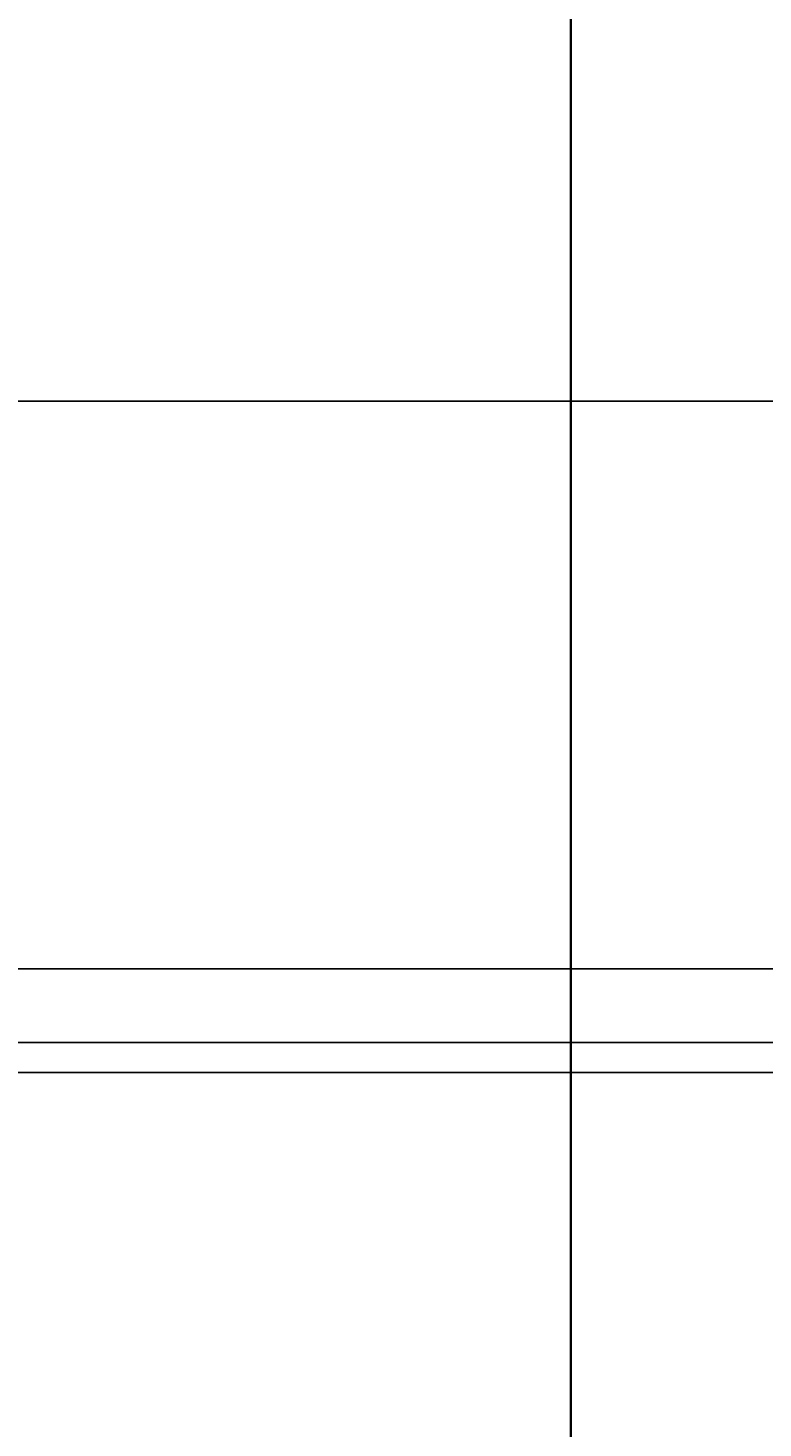
# Model space of a CAD drawing. Units: inches. Extents: x -13 to 809, y 112 to 656.
# Tile 6 of 55: x 49 to 111, y 328 to 446. Entities that reach past the tile are written whole.
import ezdxf

# ---------------------------------------------------------------- set-up
doc = ezdxf.new("R2010")
doc.units = ezdxf.units.IN
doc.header["$MEASUREMENT"] = 0
doc.layers.add('A-ANNO-DIMS', color=2, linetype='Continuous', lineweight=18)
doc.layers.add('A-ELEV', color=7, linetype='Continuous', lineweight=35)
doc.styles.get("Standard").update_dxf_attribs({"font": 'arial.ttf'})
doc.dimstyles.get("Standard").update_dxf_attribs({"dimtxt": 0.625, "dimasz": 0.18, "dimexe": 0.18, "dimexo": 0.0625, "dimgap": 0.09, "dimtad": 0, "dimtih": 1, "dimtoh": 1, "dimdec": 4, "dimzin": 0, "dimdsep": 46, "dimlunit": 4, "dimtxsty": 'Standard', "dimcen": 0.09, "dimadec": 0, "dimazin": 0, "dimtfac": 1, "dimtdec": 4, "dimtofl": 0, "dimtmove": 0, "dimatfit": 3, "dimfxl": 1, "dimtolj": 1, "dimtzin": 0, "dimarcsym": 0})

# ---------------------------------------------------------------- blocks, each defined once
blk = doc.blocks.new('*D22')
at = {"layer": 'A-ANNO-DIMS', "color": 0, "lineweight": -2, "transparency": 16777216}
for p, q in [((26.08, 210.58), (26.08, 655.96)), ((107.26, 510.58), (107.26, 655.96)), ((26.26, 655.78), (65.52, 655.78)), ((107.08, 655.78), (67.82, 655.78))]:
    blk.add_line(p, q, dxfattribs=at)
at = {"layer": 'A-ANNO-DIMS', "color": 0, "transparency": 16777216}
for points in [[(26.26, 655.81), (26.26, 655.75), (26.08, 655.78)], [(107.08, 655.81), (107.08, 655.75), (107.26, 655.78)]]:
    blk.add_solid(points, dxfattribs=at)
at = {"layer": 'Defpoints', "color": 0, "transparency": 16777216}
for p in [(107.26, 655.78), (107.26, 510.52), (26.08, 210.52)]:
    blk.add_point(p, dxfattribs=at)
at = {"layer": 'A-ANNO-DIMS', "color": 0, "transparency": 16777216, "insert": (66.67, 655.78), "char_height": 0.625, "attachment_point": 5}
blk.add_mtext('\\A1;81.18', dxfattribs=at)
blk = doc.blocks.new('*D34')
at = {"layer": 'A-ANNO-DIMS', "color": 0, "lineweight": -2, "transparency": 16777216}
for p, q in [((94.98, 462.52), (-12.1, 462.52)), ((-11.92, 462.34), (-11.92, 384.93)), ((-11.92, 306.7), (-11.92, 384.11)), ((94.98, 306.52), (-12.1, 306.52))]:
    blk.add_line(p, q, dxfattribs=at)
at = {"layer": 'A-ANNO-DIMS', "color": 0, "transparency": 16777216}
for points in [[(-11.95, 462.34), (-11.89, 462.34), (-11.92, 462.52)], [(-11.95, 306.7), (-11.89, 306.7), (-11.92, 306.52)]]:
    blk.add_solid(points, dxfattribs=at)
at = {"layer": 'Defpoints', "color": 0, "transparency": 16777216}
for p in [(-11.92, 462.52), (95.05, 462.52), (95.05, 306.52)]:
    blk.add_point(p, dxfattribs=at)
at = {"layer": 'A-ANNO-DIMS', "color": 0, "transparency": 16777216, "insert": (-11.92, 384.52), "char_height": 0.625, "attachment_point": 5}
blk.add_mtext('\\A1;156', dxfattribs=at)
blk = doc.blocks.new('*D39')
at = {"layer": 'A-ANNO-DIMS', "color": 0, "lineweight": -2, "transparency": 16777216}
for p, q in [((341.34, 524.28), (-12.1, 524.28)), ((-11.92, 524.1), (-11.92, 406.78)), ((-11.92, 288.63), (-11.92, 405.96)), ((341.34, 288.45), (-12.1, 288.45))]:
    blk.add_line(p, q, dxfattribs=at)
at = {"layer": 'A-ANNO-DIMS', "color": 0, "transparency": 16777216}
for points in [[(-11.95, 524.1), (-11.89, 524.1), (-11.92, 524.28)], [(-11.95, 288.63), (-11.89, 288.63), (-11.92, 288.45)]]:
    blk.add_solid(points, dxfattribs=at)
at = {"layer": 'Defpoints', "color": 0, "transparency": 16777216}
for p in [(-11.92, 524.28), (341.41, 524.28), (341.41, 288.45)]:
    blk.add_point(p, dxfattribs=at)
at = {"layer": 'A-ANNO-DIMS', "color": 0, "transparency": 16777216, "insert": (-11.92, 406.37), "char_height": 0.625, "attachment_point": 5}
blk.add_mtext('\\A1;235.83', dxfattribs=at)
blk = doc.blocks.new('*D41')
at = {"layer": 'A-ANNO-DIMS', "color": 0, "lineweight": -2, "transparency": 16777216}
for p, q in [((471.04, 357.98), (-12.1, 357.98)), ((-11.92, 357.8), (-11.92, 335.98)), ((-11.92, 313.35), (-11.92, 335.16)), ((471.04, 313.17), (-12.1, 313.17))]:
    blk.add_line(p, q, dxfattribs=at)
at = {"layer": 'A-ANNO-DIMS', "color": 0, "transparency": 16777216}
for points in [[(-11.95, 357.8), (-11.89, 357.8), (-11.92, 357.98)], [(-11.95, 313.35), (-11.89, 313.35), (-11.92, 313.17)]]:
    blk.add_solid(points, dxfattribs=at)
at = {"layer": 'Defpoints', "color": 0, "transparency": 16777216}
for p in [(-11.92, 357.98), (471.1, 357.98), (471.1, 313.17)]:
    blk.add_point(p, dxfattribs=at)
at = {"layer": 'A-ANNO-DIMS', "color": 0, "transparency": 16777216, "insert": (-11.92, 335.57), "char_height": 0.625, "attachment_point": 5}
blk.add_mtext('\\A1;44.81', dxfattribs=at)
blk = doc.blocks.new('*D42')
at = {"layer": 'A-ANNO-DIMS', "color": 0, "lineweight": -2, "transparency": 16777216}
for p, q in [((471.04, 414.86), (-12.1, 414.86)), ((-11.92, 414.68), (-11.92, 386.83)), ((-11.92, 358.16), (-11.92, 386.01)), ((471.04, 357.98), (-12.1, 357.98))]:
    blk.add_line(p, q, dxfattribs=at)
at = {"layer": 'A-ANNO-DIMS', "color": 0, "transparency": 16777216}
for points in [[(-11.95, 414.68), (-11.89, 414.68), (-11.92, 414.86)], [(-11.95, 358.16), (-11.89, 358.16), (-11.92, 357.98)]]:
    blk.add_solid(points, dxfattribs=at)
at = {"layer": 'Defpoints', "color": 0, "transparency": 16777216}
for p in [(-11.92, 414.86), (471.1, 414.86), (471.1, 357.98)]:
    blk.add_point(p, dxfattribs=at)
at = {"layer": 'A-ANNO-DIMS', "color": 0, "transparency": 16777216, "insert": (-11.92, 386.42), "char_height": 0.625, "attachment_point": 5}
blk.add_mtext('\\A1;56.88', dxfattribs=at)
blk = doc.blocks.new('*D43')
at = {"layer": 'A-ANNO-DIMS', "color": 0, "lineweight": -2, "transparency": 16777216}
for p, q in [((471.04, 470.88), (-12.1, 470.88)), ((-11.92, 470.7), (-11.92, 443.28)), ((-11.92, 415.04), (-11.92, 442.46)), ((471.04, 414.86), (-12.1, 414.86))]:
    blk.add_line(p, q, dxfattribs=at)
at = {"layer": 'A-ANNO-DIMS', "color": 0, "transparency": 16777216}
for points in [[(-11.95, 470.7), (-11.89, 470.7), (-11.92, 470.88)], [(-11.95, 415.04), (-11.89, 415.04), (-11.92, 414.86)]]:
    blk.add_solid(points, dxfattribs=at)
at = {"layer": 'Defpoints', "color": 0, "transparency": 16777216}
for p in [(-11.92, 470.88), (471.1, 470.88), (471.1, 414.86)]:
    blk.add_point(p, dxfattribs=at)
at = {"layer": 'A-ANNO-DIMS', "color": 0, "transparency": 16777216, "insert": (-11.92, 442.87), "char_height": 0.625, "attachment_point": 5}
blk.add_mtext('\\A1;56.02', dxfattribs=at)
blk = doc.blocks.new('*D114')
at = {"layer": 'A-ANNO-DIMS', "color": 0, "lineweight": -2, "transparency": 16777216}
for p, q in [((112.98, 366.75), (-12.1, 366.75)), ((-11.92, 366.57), (-11.92, 364.05)), ((-11.92, 360.7), (-11.92, 363.23)), ((112.98, 360.52), (-12.1, 360.52))]:
    blk.add_line(p, q, dxfattribs=at)
at = {"layer": 'A-ANNO-DIMS', "color": 0, "transparency": 16777216}
for points in [[(-11.95, 366.57), (-11.89, 366.57), (-11.92, 366.75)], [(-11.95, 360.7), (-11.89, 360.7), (-11.92, 360.52)]]:
    blk.add_solid(points, dxfattribs=at)
at = {"layer": 'Defpoints', "color": 0, "transparency": 16777216}
for p in [(113.05, 366.75), (-11.92, 360.52), (113.05, 360.52)]:
    blk.add_point(p, dxfattribs=at)
at = {"layer": 'A-ANNO-DIMS', "color": 0, "transparency": 16777216, "insert": (-11.92, 363.64), "char_height": 0.625, "attachment_point": 5}
blk.add_mtext('\\A1;6.233', dxfattribs=at)

msp = doc.modelspace()

# ---------------------------------------------------------------- linework, layer by layer
at = {"layer": 'A-ELEV'}
msp.add_line((95.0469, 318.5199), (95.0469, 462.5199), dxfattribs=at)

# ---------------------------------------------------------------- dimensions: what is measured, and where the dimension line sits
at = {"layer": 'A-ANNO-DIMS'}
dim = msp.add_linear_dim(base=(107.2588, 655.7828), p1=(26.0809, 210.5199), p2=(107.2588, 510.5199), dimstyle='Standard', override={"dimdec": 2, "dimlfac": 1, "dimrnd": 0, "dimzin": 0, "dimdsep": 46, "dimlunit": 2}, dxfattribs=at)
dim.commit()
dim.dimension.update_dxf_attribs({"geometry": '*D22', "text_midpoint": (66.6698, 655.7828)})
for base, p1, p2, override, picture, middle in [((-11.9191, 524.281), (341.4072, 288.4508), (341.4072, 524.281), {"dimdec": 2, "dimlfac": 1, "dimrnd": 0, "dimzin": 0, "dimdsep": 46, "dimlunit": 2}, '*D39', (-11.9191, 406.3659)), ((-11.9191, 470.8765), (471.0998, 414.8594), (471.0998, 470.8765), {"dimdec": 2, "dimlfac": 1, "dimrnd": 0, "dimzin": 0, "dimdsep": 46, "dimlunit": 2}, '*D43', (-11.9191, 442.8679)), ((-11.9191, 462.5199), (95.0469, 306.5199), (95.0469, 462.5199), {"dimdec": 0, "dimlfac": 1, "dimrnd": 0, "dimzin": 0, "dimdsep": 46, "dimlunit": 2}, '*D34', (-11.9191, 384.5199)), ((-11.9191, 414.8594), (471.0998, 357.9804), (471.0998, 414.8594), {"dimdec": 2, "dimlfac": 1, "dimrnd": 0, "dimzin": 0, "dimdsep": 46, "dimlunit": 2}, '*D42', (-11.9191, 386.4199)), ((-11.9191, 360.5199), (113.0469, 366.753), (113.0469, 360.5199), {"dimdec": 3, "dimlfac": 1, "dimrnd": 0, "dimzin": 0, "dimdsep": 46, "dimlunit": 2}, '*D114', (-11.9191, 363.6364)), ((-11.9191, 357.9804), (471.0998, 313.1667), (471.0998, 357.9804), {"dimdec": 2, "dimlfac": 1, "dimrnd": 0, "dimzin": 0, "dimdsep": 46, "dimlunit": 2}, '*D41', (-11.9191, 335.5735))]:
    dim = msp.add_linear_dim(base=base, p1=p1, p2=p2, angle=90, dimstyle='Standard', override=override, dxfattribs=at)
    dim.commit()
    dim.dimension.update_dxf_attribs({"geometry": picture, "text_midpoint": middle})

doc.saveas('drawing.dxf')
